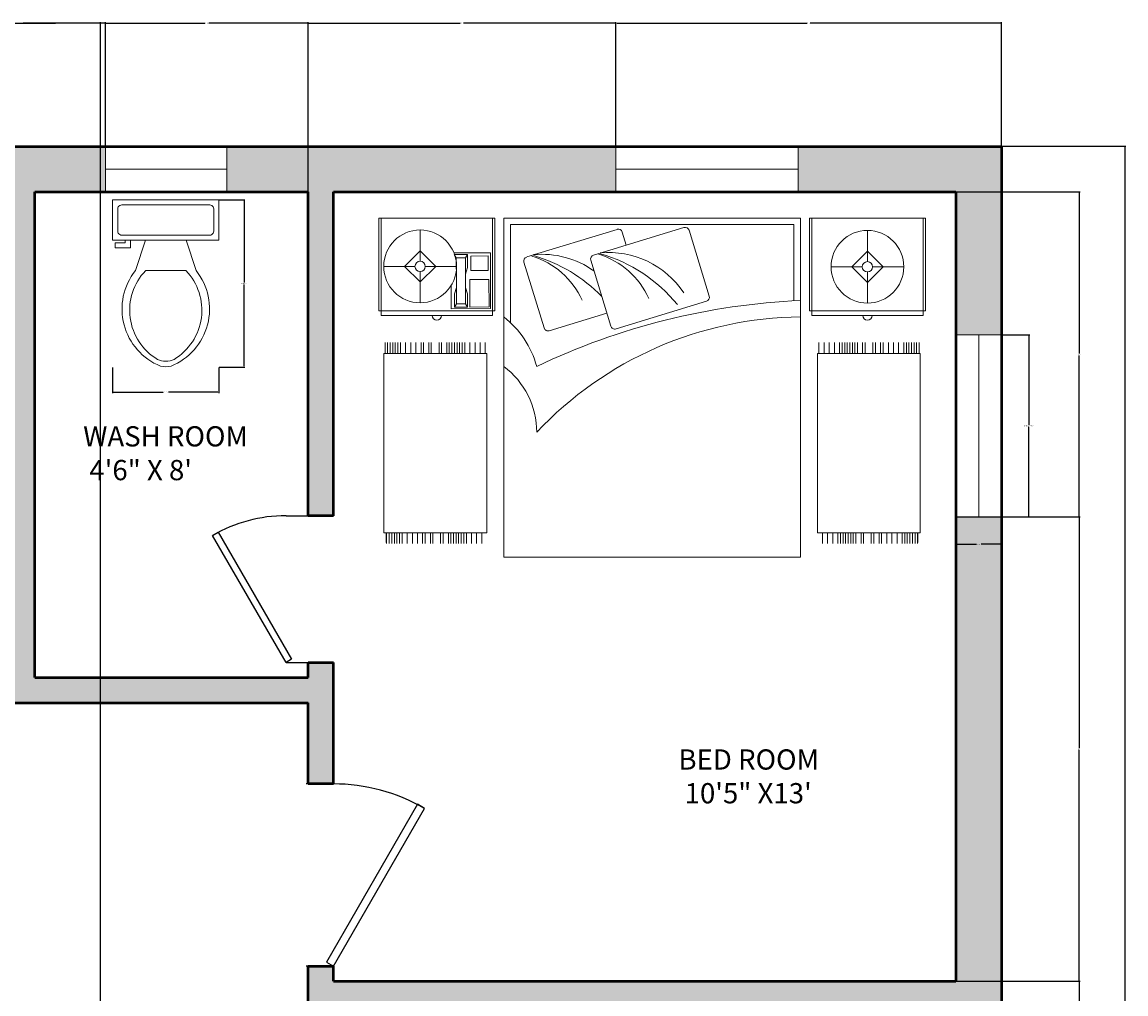
# Model space of a CAD drawing. Units: inches. Extents: x -23 to 411, y -22 to 507.
# Tile 5 of 5: x 193 to 411, y 315 to 507. Entities that reach past the tile are written whole.
import ezdxf

# ---------------------------------------------------------------- set-up
doc = ezdxf.new("R2010")
doc.units = ezdxf.units.IN
doc.header["$MEASUREMENT"] = 0
for name, color, linetype, lineweight in [('A-ANNO-DIMS', 2, 'Continuous', 18), ('A-AREA-IDEN', 7, 'Continuous', 25), ('A-FLOR-FIXT', 90, 'Continuous', 18), ('A-WALL', 7, 'Continuous', 50), ('doors', 40, 'Continuous', 25), ('furniture', 220, 'Continuous', 18), ('window', 30, 'Continuous', 18)]:
    doc.layers.add(name, color=color, linetype=linetype, lineweight=lineweight)
doc.layers.add('A-WALL-PATT', color=179, linetype='Continuous', lineweight=13, true_color=0x161b4b)
doc.styles.get("Standard").update_dxf_attribs({"font": 'arial.ttf'})
doc.dimstyles.get("Standard").update_dxf_attribs({"dimtxt": 0.18, "dimasz": 0.18, "dimexe": 0.18, "dimexo": 0.0625, "dimgap": 0.09, "dimtad": 0, "dimtih": 1, "dimtoh": 1, "dimdec": 4, "dimzin": 0, "dimdsep": 46, "dimtxsty": 'Standard', "dimcen": 0.09, "dimadec": 0, "dimazin": 0, "dimtfac": 1, "dimtdec": 4, "dimtofl": 0, "dimtmove": 0, "dimatfit": 3, "dimfxl": 1, "dimtolj": 1, "dimtzin": 0, "dimarcsym": 0})

# ---------------------------------------------------------------- blocks, each defined once
blk = doc.blocks.new('*U6')
for p, q in [((0, 0), (0, -6)), ((40, 0), (40, -6))]:
    blk.add_line(p, q)
blk.add_lwpolyline([(0, 0), (34.64, 20), (35.52, 18.48), (0.87, -1.52)], close=True)
blk.add_arc((0, 0), 40, 0, 30)
blk = doc.blocks.new('*U7')
for p, q in [((0, 0), (0, 6)), ((40, 0), (40, 6))]:
    blk.add_line(p, q)
blk.add_lwpolyline([(0, 0), (34.64, -20), (35.52, -18.48), (0.87, 1.52)], close=True)
blk.add_arc((0, 0), 40, 330, 0)
blk = doc.blocks.new('3')
for p, q in [((185.8665, 224.6766), (185.8665, 225.2363)), ((185.8665, 225.2363), (186.566, 225.2363)), ((185.8805, 224.6487), (185.8805, 225.2363)), ((186.552, 225.2363), (186.552, 224.6487)), ((186.566, 225.2363), (186.566, 224.6766)), ((186.6199, 225.2363), (186.6199, 224.6399)), ((188.4089, 225.2363), (186.6199, 225.2363)), ((188.4089, 224.7393), (188.4089, 225.2363)), ((188.4627, 225.2363), (188.4627, 224.6766)), ((189.1623, 225.2363), (188.4627, 225.2363)), ((188.4767, 225.2363), (188.4767, 224.6486)), ((189.1483, 224.6486), (189.1483, 225.2363)), ((189.1623, 224.6766), (189.1623, 225.2363)), ((186.1157, 225.1643), (186.1157, 224.9763)), ((187.3034, 225.1683), (186.7581, 225.0015)), ((187.7059, 225.1793), (187.1607, 225.0124)), ((187.3344, 225.1518), (187.3586, 225.073)), ((187.737, 225.1628), (187.8585, 224.7657)), ((188.8125, 225.1618), (188.8125, 224.9738)), ((186.0216, 224.9449), (186.1157, 225.0389)), ((186.1157, 225.0389), (186.2097, 224.9449)), ((186.5397, 225.0274), (186.3193, 225.0266)), ((186.3215, 225.0167), (186.4008, 225.017)), ((186.3334, 224.9969), (186.3215, 225.0167)), ((186.4008, 225.017), (186.389, 224.9971)), ((186.4008, 225.017), (186.4011, 224.9376)), ((186.5409, 224.6901), (186.5397, 225.0274)), ((188.8125, 225.0365), (188.7185, 224.9424)), ((188.9065, 224.9424), (188.8125, 225.0365)), ((186.0843, 224.9449), (185.8963, 224.9449)), ((186.1157, 224.8509), (186.0216, 224.9449)), ((186.2097, 224.9449), (186.1157, 224.8509)), ((186.147, 224.9449), (186.335, 224.9449)), ((186.3334, 224.9969), (186.389, 224.9971)), ((186.334, 224.858), (186.3334, 224.9969)), ((186.3895, 224.8582), (186.389, 224.9971)), ((186.7416, 224.9704), (186.8631, 224.5734)), ((187.1442, 224.9814), (187.2657, 224.5843)), ((186.1157, 224.9136), (186.1157, 224.7256)), ((186.3314, 224.9055), (186.3338, 224.8977)), ((186.4011, 224.9376), (186.3894, 224.8979)), ((188.7812, 224.9424), (188.5931, 224.9424)), ((188.7185, 224.9424), (188.8125, 224.8484)), ((188.8125, 224.8484), (188.9065, 224.9424)), ((188.8125, 224.9111), (188.8125, 224.723)), ((188.8438, 224.9424), (189.0319, 224.9424)), ((186.3023, 224.8297), (186.3029, 224.6892)), ((186.3224, 224.7786), (186.3341, 224.8183)), ((186.334, 224.858), (186.3345, 224.7191)), ((186.3895, 224.8582), (186.39, 224.7193)), ((186.4017, 224.7789), (186.3897, 224.8185)), ((186.3227, 224.6992), (186.3224, 224.7786)), ((186.402, 224.6995), (186.4017, 224.7789)), ((186.3029, 224.6892), (186.5409, 224.6901)), ((186.3345, 224.7191), (186.3227, 224.6992)), ((186.3227, 224.6992), (186.402, 224.6995)), ((186.3345, 224.7191), (186.39, 224.7193)), ((186.402, 224.6995), (186.39, 224.7193)), ((187.842, 224.7347), (187.2967, 224.5678)), ((188.4089, 224.7393), (188.4089, 223.1907)), ((186.566, 224.6766), (185.8665, 224.6766)), ((186.552, 224.6487), (185.8805, 224.6487)), ((186.6199, 224.6399), (186.6199, 223.1907)), ((187.2416, 224.6632), (186.8942, 224.5569)), ((188.4627, 224.6766), (189.1623, 224.6766)), ((188.4767, 224.6486), (189.1483, 224.6486)), ((185.904, 224.4849, -0.9094), (185.904, 224.4204, -0.9094)), ((185.9195, 224.4849, -0.9094), (185.9195, 224.4204, -0.9094)), ((185.9195, 224.4849, -0.9094), (185.9195, 224.4204, -0.9094)), ((185.935, 224.4849, -0.9094), (185.935, 224.4204, -0.9094)), ((185.9505, 224.4849, -0.9094), (185.9505, 224.4204, -0.9094)), ((185.966, 224.4849, -0.9094), (185.966, 224.4204, -0.9094)), ((185.9815, 224.4849, -0.9094), (185.9815, 224.4204, -0.9094)), ((185.997, 224.4849, -0.9094), (185.997, 224.4204, -0.9094)), ((186.028, 224.4849, -0.9094), (186.028, 224.4204, -0.9094)), ((186.059, 224.4849, -0.9094), (186.059, 224.4204, -0.9094)), ((186.09, 224.4849, -0.9094), (186.09, 224.4204, -0.9094)), ((186.09, 224.4849, -0.9094), (186.09, 224.4204, -0.9094)), ((186.121, 224.4849, -0.9094), (186.121, 224.4204, -0.9094)), ((186.1365, 224.4849, -0.9094), (186.1365, 224.4204, -0.9094)), ((186.1675, 224.4849, -0.9094), (186.1675, 224.4204, -0.9094)), ((186.183, 224.4849, -0.9094), (186.183, 224.4204, -0.9094)), ((186.2295, 224.4849, -0.9094), (186.2295, 224.4204, -0.9094)), ((186.245, 224.4849, -0.9094), (186.245, 224.4204, -0.9094)), ((186.276, 224.4849, -0.9094), (186.276, 224.4204, -0.9094)), ((186.2915, 224.4849, -0.9094), (186.2915, 224.4204, -0.9094)), ((186.307, 224.4849, -0.9094), (186.307, 224.4204, -0.9094)), ((186.3225, 224.4849, -0.9094), (186.3225, 224.4204, -0.9094)), ((186.338, 224.4849, -0.9094), (186.338, 224.4204, -0.9094)), ((186.3535, 224.4849, -0.9094), (186.3535, 224.4204, -0.9094)), ((186.369, 224.4849, -0.9094), (186.369, 224.4204, -0.9094)), ((186.3845, 224.4849, -0.9094), (186.3845, 224.4204, -0.9094)), ((186.4155, 224.4849, -0.9094), (186.4155, 224.4204, -0.9094)), ((186.4465, 224.4849, -0.9094), (186.4465, 224.4204, -0.9094)), ((186.4775, 224.4849, -0.9094), (186.4775, 224.4204, -0.9094)), ((186.5085, 224.4849, -0.9094), (186.5085, 224.4204, -0.9094)), ((188.5202, 224.4849, -0.9094), (188.5202, 224.4204, -0.9094)), ((188.5512, 224.4849, -0.9094), (188.5512, 224.4204, -0.9094)), ((188.5822, 224.4849, -0.9094), (188.5822, 224.4204, -0.9094)), ((188.6132, 224.4849, -0.9094), (188.6132, 224.4204, -0.9094)), ((188.6442, 224.4849, -0.9094), (188.6442, 224.4204, -0.9094)), ((188.6597, 224.4849, -0.9094), (188.6597, 224.4204, -0.9094)), ((188.6752, 224.4849, -0.9094), (188.6752, 224.4204, -0.9094)), ((188.6907, 224.4849, -0.9094), (188.6907, 224.4204, -0.9094)), ((188.7062, 224.4849, -0.9094), (188.7062, 224.4204, -0.9094)), ((188.7217, 224.4849, -0.9094), (188.7217, 224.4204, -0.9094)), ((188.7372, 224.4849, -0.9094), (188.7372, 224.4204, -0.9094)), ((188.7527, 224.4849, -0.9094), (188.7527, 224.4204, -0.9094)), ((188.7837, 224.4849, -0.9094), (188.7837, 224.4204, -0.9094)), ((188.7992, 224.4849, -0.9094), (188.7992, 224.4204, -0.9094)), ((188.8457, 224.4849, -0.9094), (188.8457, 224.4204, -0.9094)), ((188.8612, 224.4849, -0.9094), (188.8612, 224.4204, -0.9094)), ((188.8922, 224.4849, -0.9094), (188.8922, 224.4204, -0.9094)), ((188.9077, 224.4849, -0.9094), (188.9077, 224.4204, -0.9094)), ((188.9387, 224.4849, -0.9094), (188.9387, 224.4204, -0.9094)), ((188.9387, 224.4849, -0.9094), (188.9387, 224.4204, -0.9094)), ((188.9697, 224.4849, -0.9094), (188.9697, 224.4204, -0.9094)), ((189.0007, 224.4849, -0.9094), (189.0007, 224.4204, -0.9094)), ((189.0317, 224.4849, -0.9094), (189.0317, 224.4204, -0.9094)), ((189.0472, 224.4849, -0.9094), (189.0472, 224.4204, -0.9094)), ((189.0627, 224.4849, -0.9094), (189.0627, 224.4204, -0.9094)), ((189.0782, 224.4849, -0.9094), (189.0782, 224.4204, -0.9094)), ((189.0937, 224.4849, -0.9094), (189.0937, 224.4204, -0.9094)), ((189.1092, 224.4849, -0.9094), (189.1092, 224.4204, -0.9094)), ((189.1092, 224.4849, -0.9094), (189.1092, 224.4204, -0.9094)), ((189.1247, 224.4849, -0.9094), (189.1247, 224.4204, -0.9094)), ((185.8974, 224.4204, -0.9094), (185.8974, 223.3378, -0.9094)), ((185.8974, 224.4204, -0.9094), (186.5174, 224.4204, -0.9094)), ((186.5174, 224.4204, -0.9094), (186.5174, 223.3378, -0.9094)), ((189.1313, 224.4204, -0.9094), (188.5113, 224.4204, -0.9094)), ((188.5113, 224.4204, -0.9094), (188.5113, 223.3378, -0.9094)), ((189.1313, 224.4204, -0.9094), (189.1313, 223.3378, -0.9094)), ((185.8974, 223.3378, -0.9094), (186.5174, 223.3378, -0.9094)), ((185.9114, 223.3378, -0.9094), (185.9114, 223.2789, -0.9094)), ((185.9114, 223.3378, -0.9094), (185.9114, 223.2789, -0.9094)), ((185.9114, 223.3378, -0.9094), (185.9114, 223.2789, -0.9094)), ((185.9138, 223.3378, -0.9094), (185.9138, 223.2732, -0.9094)), ((185.9293, 223.3378, -0.9094), (185.9293, 223.2732, -0.9094)), ((185.9293, 223.3378, -0.9094), (185.9293, 223.2732, -0.9094)), ((185.9448, 223.3378, -0.9094), (185.9448, 223.2732, -0.9094)), ((185.9603, 223.3378, -0.9094), (185.9603, 223.2732, -0.9094)), ((185.9758, 223.3378, -0.9094), (185.9758, 223.2732, -0.9094)), ((185.9913, 223.3378, -0.9094), (185.9913, 223.2732, -0.9094)), ((186.0068, 223.3378, -0.9094), (186.0068, 223.2732, -0.9094)), ((186.0378, 223.3378, -0.9094), (186.0378, 223.2732, -0.9094)), ((186.0688, 223.3378, -0.9094), (186.0688, 223.2732, -0.9094)), ((186.0998, 223.3378, -0.9094), (186.0998, 223.2732, -0.9094)), ((186.0998, 223.3378, -0.9094), (186.0998, 223.2732, -0.9094)), ((186.1308, 223.3378, -0.9094), (186.1308, 223.2732, -0.9094)), ((186.1463, 223.3378, -0.9094), (186.1463, 223.2732, -0.9094)), ((186.1773, 223.3378, -0.9094), (186.1773, 223.2732, -0.9094)), ((186.1928, 223.3378, -0.9094), (186.1928, 223.2732, -0.9094)), ((186.2393, 223.3378, -0.9094), (186.2393, 223.2732, -0.9094)), ((186.2548, 223.3378, -0.9094), (186.2548, 223.2732, -0.9094)), ((186.2858, 223.3378, -0.9094), (186.2858, 223.2732, -0.9094)), ((186.3013, 223.3378, -0.9094), (186.3013, 223.2732, -0.9094)), ((186.3168, 223.3378, -0.9094), (186.3168, 223.2732, -0.9094)), ((186.3323, 223.3378, -0.9094), (186.3323, 223.2732, -0.9094)), ((186.3478, 223.3378, -0.9094), (186.3478, 223.2732, -0.9094)), ((186.3633, 223.3378, -0.9094), (186.3633, 223.2732, -0.9094)), ((186.3788, 223.3378, -0.9094), (186.3788, 223.2732, -0.9094)), ((186.3943, 223.3378, -0.9094), (186.3943, 223.2732, -0.9094)), ((186.4253, 223.3378, -0.9094), (186.4253, 223.2732, -0.9094)), ((186.4563, 223.3378, -0.9094), (186.4563, 223.2732, -0.9094)), ((186.4873, 223.3378, -0.9094), (186.4873, 223.2732, -0.9094)), ((189.1313, 223.3378, -0.9094), (188.5113, 223.3378, -0.9094)), ((188.5414, 223.3378, -0.9094), (188.5414, 223.2732, -0.9094)), ((188.5724, 223.3378, -0.9094), (188.5724, 223.2732, -0.9094)), ((188.6034, 223.3378, -0.9094), (188.6034, 223.2732, -0.9094)), ((188.6344, 223.3378, -0.9094), (188.6344, 223.2732, -0.9094)), ((188.6499, 223.3378, -0.9094), (188.6499, 223.2732, -0.9094)), ((188.6654, 223.3378, -0.9094), (188.6654, 223.2732, -0.9094)), ((188.6809, 223.3378, -0.9094), (188.6809, 223.2732, -0.9094)), ((188.6964, 223.3378, -0.9094), (188.6964, 223.2732, -0.9094)), ((188.7119, 223.3378, -0.9094), (188.7119, 223.2732, -0.9094)), ((188.7274, 223.3378, -0.9094), (188.7274, 223.2732, -0.9094)), ((188.7429, 223.3378, -0.9094), (188.7429, 223.2732, -0.9094)), ((188.7739, 223.3378, -0.9094), (188.7739, 223.2732, -0.9094)), ((188.7894, 223.3378, -0.9094), (188.7894, 223.2732, -0.9094)), ((188.8359, 223.3378, -0.9094), (188.8359, 223.2732, -0.9094)), ((188.8514, 223.3378, -0.9094), (188.8514, 223.2732, -0.9094)), ((188.8824, 223.3378, -0.9094), (188.8824, 223.2732, -0.9094)), ((188.8979, 223.3378, -0.9094), (188.8979, 223.2732, -0.9094)), ((188.9289, 223.3378, -0.9094), (188.9289, 223.2732, -0.9094)), ((188.9289, 223.3378, -0.9094), (188.9289, 223.2732, -0.9094)), ((188.9599, 223.3378, -0.9094), (188.9599, 223.2732, -0.9094)), ((188.9909, 223.3378, -0.9094), (188.9909, 223.2732, -0.9094)), ((189.022, 223.3378, -0.9094), (189.022, 223.2732, -0.9094)), ((189.0375, 223.3378, -0.9094), (189.0375, 223.2732, -0.9094)), ((189.053, 223.3378, -0.9094), (189.053, 223.2732, -0.9094)), ((189.0685, 223.3378, -0.9094), (189.0685, 223.2732, -0.9094)), ((189.084, 223.3378, -0.9094), (189.084, 223.2732, -0.9094)), ((189.0995, 223.3378, -0.9094), (189.0995, 223.2732, -0.9094)), ((189.0995, 223.3378, -0.9094), (189.0995, 223.2732, -0.9094)), ((189.115, 223.3378, -0.9094), (189.115, 223.2732, -0.9094)), ((189.1173, 223.3378, -0.9094), (189.1173, 223.2789, -0.9094)), ((189.1173, 223.3378, -0.9094), (189.1173, 223.2789, -0.9094)), ((189.1173, 223.3378, -0.9094), (189.1173, 223.2789, -0.9094)), ((186.6199, 223.1907), (188.4089, 223.1907))]:
    blk.add_line(p, q)
blk.add_lwpolyline([(188.3691, 224.7374), (188.3691, 225.1965), (186.6596, 225.1965), (186.6596, 224.606)])
for points in [[(186.4217, 225.0072), (186.422, 224.9199), (186.5252, 224.9202), (186.5249, 225.0075)], [(186.4153, 224.8663), (186.4159, 224.6996), (186.531, 224.7), (186.5304, 224.8667)]]:
    blk.add_lwpolyline(points, close=True)
for points in [[(186.6199, 224.6399, -0.162278), (186.8186, 224.3418, -0.100664), (188.4089, 224.7393, -0.100664)], [(186.6199, 224.3418, -0.236068), (186.8186, 223.9442, -0.205258), (188.4089, 224.6399, -0.205258)]]:
    blk.add_lwpolyline(points, format="xyb")
for centre, radius in [((186.1157, 224.9449), 0.2194), ((188.8125, 224.9424), 0.2194), ((186.1157, 224.9449), 0.0313), ((188.8125, 224.9424), 0.0313)]:
    blk.add_circle(centre, radius)
for centre, radius, start, end in [((187.3107, 225.1446), 0.0248, 17.0142, 107.0142), ((187.7132, 225.1555), 0.0248, 17.0142, 107.0142), ((186.8477, 224.4712), 0.5468, 54.68511, 95.16051), ((187.1679, 224.9887), 0.0248, 107.0142, 197.0142), ((187.0499, 224.5517), 0.4873, 24.22087, 73.06906), ((187.2502, 224.4821), 0.5468, 33.78007, 95.16051), ((186.9385, 224.1164), 0.9426, 39.40233, 73.71889), ((186.7654, 224.9777), 0.0248, 107.0142, 197.0142), ((186.6474, 224.5408), 0.4873, 24.22087, 73.06906), ((186.5359, 224.1054), 0.9426, 44.27274, 73.71889), ((187.8347, 224.7585), 0.0248, 287.0142, 17.0142), ((186.2163, 224.6487), 0.028, 180, 0), ((188.8125, 224.6486), 0.028, 180, 0), ((186.8869, 224.5806), 0.0248, 197.0142, 287.0142), ((187.2894, 224.5916), 0.0248, 197.0142, 287.0142)]:
    blk.add_arc(centre, radius, start, end)
blk = doc.blocks.new('Toilet - top')
for p, q in [((9.5, -6), (9.5, -2)), ((-10, -8.5), (-8, -8.5)), ((-10, -9.5), (-10, -8.5)), ((-8, -8.5), (-8, -8)), ((-7, -8), (-7, -9.5)), ((-4, -8), (-6, -14)), ((4, -8), (6, -14)), ((-7, -9.5), (-10, -9.5)), ((4, -14), (-4, -14))]:
    blk.add_line(p, q)
blk.add_lwpolyline([(10.5, -8), (10.5, 0), (-10.5, 0), (-10.5, -8)], close=True)
for points in [[(-9.5, -2), (-9.5, -6)], [(8.5, -1), (-8.5, -1)], [(-8.5, -7), (8.5, -7)]]:
    blk.add_lwpolyline(points)
for centre, radius, start, end in [((-8.62, -1.88), 0.884, 81.8699, 188.1301), ((8.62, -1.88), 0.884, 351.8699, 98.1301), ((-8.62, -6.12), 0.884, 171.8699, 278.1301), ((8.62, -6.12), 0.884, 261.8699, 8.1301), ((3.52, -21.58), 12.17, 141.4691, 247.9714), ((4.2, -21.82), 11.33, 136.3677, 238.9468), ((-3.52, -21.58), 12.17, 292.0284, 38.5307), ((-4.2, -21.82), 11.33, 301.053, 43.6321), ((0, -27.88), 4, 245.7318, 294.2682), ((0, -29), 4, 254.8605, 285.1395)]:
    blk.add_arc(centre, radius, start, end)
blk = doc.blocks.new('WIN-36IN')
for p, q in [((9, 36), (0, 36)), ((0, 36), (0, 0)), ((4.5, 0), (4.5, 36)), ((9, 0), (9, 36)), ((0, 0), (9, 0)), ((0, 0), (4.5, 0))]:
    blk.add_line(p, q)
blk = doc.blocks.new('WIN-24IN')
for p, q in [((0, 9), (0, 0)), ((24, 9), (0, 9)), ((0, 9), (0, 4.5)), ((24, 0), (24, 9)), ((0, 4.5), (24, 4.5)), ((0, 0), (24, 0))]:
    blk.add_line(p, q)
blk = doc.blocks.new('*D12')
at = {"layer": 'A-ANNO-DIMS', "color": 0, "lineweight": -2, "transparency": 16777216}
for p, q in [((386.24, 445.65), (391.75, 445.65)), ((391.57, 445.47), (391.57, 427.83)), ((391.57, 409.83), (391.57, 427.46)), ((386.24, 409.65), (391.75, 409.65))]:
    blk.add_line(p, q, dxfattribs=at)
at = {"layer": 'A-ANNO-DIMS', "color": 0, "transparency": 16777216}
for points in [[(391.54, 445.47), (391.6, 445.47), (391.57, 445.65)], [(391.54, 409.83), (391.6, 409.83), (391.57, 409.65)]]:
    blk.add_solid(points, dxfattribs=at)
at = {"layer": 'Defpoints', "color": 0, "transparency": 16777216}
for p in [(386.17, 445.65), (391.57, 445.65), (386.17, 409.65)]:
    blk.add_point(p, dxfattribs=at)
at = {"layer": 'A-ANNO-DIMS', "color": 0, "transparency": 16777216, "insert": (391.57, 427.65), "char_height": 0.18, "attachment_point": 5}
blk.add_mtext('\\A1;WINDOW 36 TYP.', dxfattribs=at)
blk = doc.blocks.new('*D13')
at = {"layer": 'A-ANNO-DIMS', "color": 0, "lineweight": -2, "transparency": 16777216}
for p, q in [((377.17, 409.58), (377.17, 404.07)), ((386.17, 409.58), (386.17, 404.07)), ((377.35, 404.25), (381.22, 404.25)), ((385.99, 404.25), (382.13, 404.25))]:
    blk.add_line(p, q, dxfattribs=at)
at = {"layer": 'A-ANNO-DIMS', "color": 0, "transparency": 16777216}
for points in [[(377.35, 404.28), (377.35, 404.22), (377.17, 404.25)], [(385.99, 404.28), (385.99, 404.22), (386.17, 404.25)]]:
    blk.add_solid(points, dxfattribs=at)
at = {"layer": 'Defpoints', "color": 0, "transparency": 16777216}
for p in [(377.17, 409.65), (386.17, 409.65), (386.17, 404.25)]:
    blk.add_point(p, dxfattribs=at)
at = {"layer": 'A-ANNO-DIMS', "color": 0, "transparency": 16777216, "insert": (381.67, 404.25), "char_height": 0.18, "attachment_point": 5}
blk.add_mtext('\\A1;9 TYP.', dxfattribs=at)
blk = doc.blocks.new('*D18')
at = {"layer": 'A-ANNO-DIMS', "color": 0, "lineweight": -2, "transparency": 16777216}
for p, q in [((231.63, 472.33), (236.7, 472.33)), ((236.52, 472.15), (236.52, 455.99)), ((236.52, 439.46), (236.52, 455.62)), ((231.63, 439.28), (236.7, 439.28))]:
    blk.add_line(p, q, dxfattribs=at)
at = {"layer": 'A-ANNO-DIMS', "color": 0, "transparency": 16777216}
for points in [[(236.49, 472.15), (236.55, 472.15), (236.52, 472.33)], [(236.49, 439.46), (236.55, 439.46), (236.52, 439.28)]]:
    blk.add_solid(points, dxfattribs=at)
at = {"layer": 'Defpoints', "color": 0, "transparency": 16777216}
for p in [(231.56, 472.33), (236.52, 472.33), (231.56, 439.28)]:
    blk.add_point(p, dxfattribs=at)
at = {"layer": 'A-ANNO-DIMS', "color": 0, "transparency": 16777216, "insert": (236.52, 455.8), "char_height": 0.18, "attachment_point": 5}
blk.add_mtext('\\A1;WC 33 TYP.', dxfattribs=at)
blk = doc.blocks.new('*D19')
at = {"layer": 'A-ANNO-DIMS', "color": 0, "lineweight": -2, "transparency": 16777216}
for p, q in [((210.56, 439.22), (210.56, 434.14)), ((231.56, 439.22), (231.56, 434.14)), ((210.74, 434.32), (220.53, 434.32)), ((231.38, 434.32), (221.59, 434.32))]:
    blk.add_line(p, q, dxfattribs=at)
at = {"layer": 'A-ANNO-DIMS', "color": 0, "transparency": 16777216}
for points in [[(210.74, 434.35), (210.74, 434.29), (210.56, 434.32)], [(231.38, 434.35), (231.38, 434.29), (231.56, 434.32)]]:
    blk.add_solid(points, dxfattribs=at)
at = {"layer": 'Defpoints', "color": 0, "transparency": 16777216}
for p in [(210.56, 439.28), (231.56, 439.28), (231.56, 434.32)]:
    blk.add_point(p, dxfattribs=at)
at = {"layer": 'A-ANNO-DIMS', "color": 0, "transparency": 16777216, "insert": (221.06, 434.32), "char_height": 0.18, "attachment_point": 5}
blk.add_mtext('\\A1;21 TYP.', dxfattribs=at)
blk = doc.blocks.new('*D29')
at = {"layer": 'A-ANNO-DIMS', "color": 0, "lineweight": -2, "transparency": 16777216}
for p, q in [((386.24, 482.9), (410.73, 482.9)), ((410.55, 482.72), (410.55, 243.08)), ((410.55, 3.08), (410.55, 242.72)), ((386.24, 2.9), (410.73, 2.9))]:
    blk.add_line(p, q, dxfattribs=at)
at = {"layer": 'A-ANNO-DIMS', "color": 0, "transparency": 16777216}
for points in [[(410.52, 482.72), (410.58, 482.72), (410.55, 482.9)], [(410.52, 3.08), (410.58, 3.08), (410.55, 2.9)]]:
    blk.add_solid(points, dxfattribs=at)
at = {"layer": 'Defpoints', "color": 0, "transparency": 16777216}
for p in [(386.17, 482.9), (386.17, 2.9), (410.55, 2.9)]:
    blk.add_point(p, dxfattribs=at)
at = {"layer": 'A-ANNO-DIMS', "color": 0, "transparency": 16777216, "insert": (410.55, 242.9), "char_height": 0.18, "attachment_point": 5}
blk.add_mtext('\\A1;480', dxfattribs=at)
blk = doc.blocks.new('*D34')
at = {"layer": 'A-ANNO-DIMS', "color": 0, "lineweight": -2, "transparency": 16777216}
for p, q in [((190.17, 473.96), (190.17, 507.45)), ((190.35, 507.27), (199.27, 507.27)), ((208.96, 507.27), (200.04, 507.27)), ((209.14, 482.96), (209.14, 507.45))]:
    blk.add_line(p, q, dxfattribs=at)
at = {"layer": 'A-ANNO-DIMS', "color": 0, "transparency": 16777216}
for points in [[(190.35, 507.3), (190.35, 507.24), (190.17, 507.27)], [(208.96, 507.3), (208.96, 507.24), (209.14, 507.27)]]:
    blk.add_solid(points, dxfattribs=at)
at = {"layer": 'Defpoints', "color": 0, "transparency": 16777216}
for p in [(209.14, 507.27), (209.14, 482.9), (190.17, 473.9)]:
    blk.add_point(p, dxfattribs=at)
at = {"layer": 'A-ANNO-DIMS', "color": 0, "transparency": 16777216, "insert": (199.66, 507.27), "char_height": 0.18, "attachment_point": 5}
blk.add_mtext('\\A1;18.96', dxfattribs=at)
blk = doc.blocks.new('*D35')
at = {"layer": 'A-ANNO-DIMS', "color": 0, "lineweight": -2, "transparency": 16777216}
for p, q in [((209.14, 482.96), (209.14, 507.45)), ((209.32, 507.27), (228.76, 507.27)), ((248.99, 507.27), (229.55, 507.27)), ((249.17, 473.96), (249.17, 507.45))]:
    blk.add_line(p, q, dxfattribs=at)
at = {"layer": 'A-ANNO-DIMS', "color": 0, "transparency": 16777216}
for points in [[(209.32, 507.3), (209.32, 507.24), (209.14, 507.27)], [(248.99, 507.3), (248.99, 507.24), (249.17, 507.27)]]:
    blk.add_solid(points, dxfattribs=at)
at = {"layer": 'Defpoints', "color": 0, "transparency": 16777216}
for p in [(249.17, 507.27), (209.14, 482.9), (249.17, 473.9)]:
    blk.add_point(p, dxfattribs=at)
at = {"layer": 'A-ANNO-DIMS', "color": 0, "transparency": 16777216, "insert": (229.16, 507.27), "char_height": 0.18, "attachment_point": 5}
blk.add_mtext('\\A1;40.04', dxfattribs=at)
blk = doc.blocks.new('*D36')
at = {"layer": 'A-ANNO-DIMS', "color": 0, "lineweight": -2, "transparency": 16777216}
for p, q in [((249.17, 473.96), (249.17, 507.45)), ((249.35, 507.27), (279.25, 507.27)), ((309.79, 507.27), (279.9, 507.27)), ((309.97, 482.96), (309.97, 507.45))]:
    blk.add_line(p, q, dxfattribs=at)
at = {"layer": 'A-ANNO-DIMS', "color": 0, "transparency": 16777216}
for points in [[(249.35, 507.3), (249.35, 507.24), (249.17, 507.27)], [(309.79, 507.3), (309.79, 507.24), (309.97, 507.27)]]:
    blk.add_solid(points, dxfattribs=at)
at = {"layer": 'Defpoints', "color": 0, "transparency": 16777216}
for p in [(309.97, 507.27), (309.97, 482.9), (249.17, 473.9)]:
    blk.add_point(p, dxfattribs=at)
at = {"layer": 'A-ANNO-DIMS', "color": 0, "transparency": 16777216, "insert": (279.57, 507.27), "char_height": 0.18, "attachment_point": 5}
blk.add_mtext('\\A1;60.8', dxfattribs=at)
blk = doc.blocks.new('*D37')
at = {"layer": 'A-ANNO-DIMS', "color": 0, "lineweight": -2, "transparency": 16777216}
for p, q in [((309.97, 482.96), (309.97, 507.45)), ((310.15, 507.27), (347.75, 507.27)), ((385.99, 507.27), (348.4, 507.27)), ((386.17, 482.96), (386.17, 507.45))]:
    blk.add_line(p, q, dxfattribs=at)
at = {"layer": 'A-ANNO-DIMS', "color": 0, "transparency": 16777216}
for points in [[(310.15, 507.3), (310.15, 507.24), (309.97, 507.27)], [(385.99, 507.3), (385.99, 507.24), (386.17, 507.27)]]:
    blk.add_solid(points, dxfattribs=at)
at = {"layer": 'Defpoints', "color": 0, "transparency": 16777216}
for p in [(386.17, 507.27), (309.97, 482.9), (386.17, 482.9)]:
    blk.add_point(p, dxfattribs=at)
at = {"layer": 'A-ANNO-DIMS', "color": 0, "transparency": 16777216, "insert": (348.07, 507.27), "char_height": 0.18, "attachment_point": 5}
blk.add_mtext('\\A1;76.2', dxfattribs=at)
blk = doc.blocks.new('*D46')
at = {"layer": 'A-ANNO-DIMS', "color": 0, "lineweight": -2, "transparency": 16777216}
for p, q in [((177.17, 107.96), (177.17, 507.45)), ((177.35, 507.27), (192.47, 507.27)), ((207.99, 507.27), (192.88, 507.27)), ((208.17, 107.96), (208.17, 507.45))]:
    blk.add_line(p, q, dxfattribs=at)
at = {"layer": 'A-ANNO-DIMS', "color": 0, "transparency": 16777216}
for points in [[(177.35, 507.3), (177.35, 507.24), (177.17, 507.27)], [(207.99, 507.3), (207.99, 507.24), (208.17, 507.27)]]:
    blk.add_solid(points, dxfattribs=at)
at = {"layer": 'Defpoints', "color": 0, "transparency": 16777216}
for p in [(208.17, 507.27), (177.17, 107.9), (208.17, 107.9)]:
    blk.add_point(p, dxfattribs=at)
at = {"layer": 'A-ANNO-DIMS', "color": 0, "transparency": 16777216, "insert": (192.67, 507.27), "char_height": 0.18, "attachment_point": 5}
blk.add_mtext('\\A1;31', dxfattribs=at)
blk = doc.blocks.new('*D55')
at = {"layer": 'A-ANNO-DIMS', "color": 0, "lineweight": -2, "transparency": 16777216}
for p, q in [((377.24, 317.9), (401.73, 317.9)), ((401.55, 317.72), (401.55, 281.82)), ((401.55, 245.55), (401.55, 281.45)), ((377.24, 245.37), (401.73, 245.37))]:
    blk.add_line(p, q, dxfattribs=at)
at = {"layer": 'A-ANNO-DIMS', "color": 0, "transparency": 16777216}
for points in [[(401.52, 317.72), (401.58, 317.72), (401.55, 317.9)], [(401.52, 245.55), (401.58, 245.55), (401.55, 245.37)]]:
    blk.add_solid(points, dxfattribs=at)
at = {"layer": 'Defpoints', "color": 0, "transparency": 16777216}
for p in [(377.17, 317.9), (377.17, 245.37), (401.55, 245.37)]:
    blk.add_point(p, dxfattribs=at)
at = {"layer": 'A-ANNO-DIMS', "color": 0, "transparency": 16777216, "insert": (401.55, 281.64), "char_height": 0.18, "attachment_point": 5}
blk.add_mtext('\\A1;72.52', dxfattribs=at)
blk = doc.blocks.new('*D56')
at = {"layer": 'A-ANNO-DIMS', "color": 0, "lineweight": -2, "transparency": 16777216}
for p, q in [((377.24, 409.65), (401.73, 409.65)), ((401.55, 409.47), (401.55, 363.95)), ((401.55, 318.08), (401.55, 363.59)), ((377.24, 317.9), (401.73, 317.9))]:
    blk.add_line(p, q, dxfattribs=at)
at = {"layer": 'A-ANNO-DIMS', "color": 0, "transparency": 16777216}
for points in [[(401.52, 409.47), (401.58, 409.47), (401.55, 409.65)], [(401.52, 318.08), (401.58, 318.08), (401.55, 317.9)]]:
    blk.add_solid(points, dxfattribs=at)
at = {"layer": 'Defpoints', "color": 0, "transparency": 16777216}
for p in [(377.17, 409.65), (377.17, 317.9), (401.55, 317.9)]:
    blk.add_point(p, dxfattribs=at)
at = {"layer": 'A-ANNO-DIMS', "color": 0, "transparency": 16777216, "insert": (401.55, 363.77), "char_height": 0.18, "attachment_point": 5}
blk.add_mtext('\\A1;91.75', dxfattribs=at)
blk = doc.blocks.new('*D57')
at = {"layer": 'A-ANNO-DIMS', "color": 0, "lineweight": -2, "transparency": 16777216}
for p, q in [((377.24, 473.9), (401.73, 473.9)), ((401.55, 473.72), (401.55, 441.95)), ((401.55, 409.83), (401.55, 441.59)), ((377.24, 409.65), (401.73, 409.65))]:
    blk.add_line(p, q, dxfattribs=at)
at = {"layer": 'A-ANNO-DIMS', "color": 0, "transparency": 16777216}
for points in [[(401.52, 473.72), (401.58, 473.72), (401.55, 473.9)], [(401.52, 409.83), (401.58, 409.83), (401.55, 409.65)]]:
    blk.add_solid(points, dxfattribs=at)
at = {"layer": 'Defpoints', "color": 0, "transparency": 16777216}
for p in [(377.17, 473.9), (377.17, 409.65), (401.55, 409.65)]:
    blk.add_point(p, dxfattribs=at)
at = {"layer": 'A-ANNO-DIMS', "color": 0, "transparency": 16777216, "insert": (401.55, 441.77), "char_height": 0.18, "attachment_point": 5}
blk.add_mtext('\\A1;64.25', dxfattribs=at)

msp = doc.modelspace()

# ---------------------------------------------------------------- hatches: boundary and pattern name
at = {"layer": 'A-WALL-PATT'}
h = msp.add_hatch(color=256, dxfattribs=at)
h.dxf.hatch_style = 1
h.paths.add_polyline_path([(37.3453, 482.8972), (2.1746, 482.8972), (2.1746, 414.9823), (11.1746, 414.9823), (11.1746, 473.8972), (37.3453, 473.8972)])
h.paths.add_polyline_path([(149.2817, 482.8972), (73.3453, 482.8972), (73.3453, 473.8972), (131.1746, 473.8972), (131.1746, 356.8972), (136.1746, 356.8972), (136.1746, 372.8972), (139.1746, 372.8972), (139.1746, 377.8972), (136.1746, 377.8972), (136.1746, 473.8972), (149.2817, 473.8972)])
h.paths.add_polyline_path([(209.1361, 482.8972), (173.2817, 482.8972), (173.2817, 473.8972), (190.1746, 473.8972), (190.1746, 377.8972), (168.1746, 377.8972), (168.1746, 372.8972), (249.1746, 372.8972), (249.1746, 356.8972), (254.1746, 356.8972), (254.1746, 380.8972), (249.1746, 380.8972), (249.1746, 377.8972), (195.1746, 377.8972), (195.1746, 473.8972), (209.1361, 473.8972)])
h.paths.add_polyline_path([(309.9724, 482.8972), (233.1361, 482.8972), (233.1361, 473.8972), (249.1746, 473.8972), (249.1746, 409.8972), (254.1746, 409.8972), (254.1746, 473.8972), (309.9724, 473.8972)])
h.paths.add_polyline_path([(386.1746, 482.8972), (345.9724, 482.8972), (345.9724, 473.8972), (377.1746, 473.8972), (377.1746, 445.6454), (386.1746, 445.6454)])
h.paths.add_polyline_path([(386.1746, 409.6454), (377.1746, 409.6454), (377.1746, 317.8972), (254.1746, 317.8972), (254.1746, 320.8972), (249.1746, 320.8972), (249.1746, 317.8972), (249.1746, 235.8972), (254.1746, 235.8972), (254.1746, 312.8972), (377.1746, 312.8972), (377.1746, 281.3732), (386.1746, 281.3732)])
h.paths.add_polyline_path([(386.1746, 245.3732), (377.1746, 245.3732), (377.1746, 196.8972), (254.1746, 196.8972), (254.1746, 199.8972), (249.1746, 199.8972), (249.1746, 196.8972), (249.1746, 188.8972), (254.1746, 188.8972), (254.1746, 191.8972), (264.1746, 191.8972), (377.1746, 191.8972), (377.1746, 11.8972), (377.1746, 2.8972), (386.1746, 2.8972)])
h.paths.add_polyline_path([(254.1746, 128.8972), (249.1746, 128.8972), (249.1746, 11.8972), (206.9157, 11.8972), (206.9157, 2.8972), (254.1746, 2.8972)])
h.paths.add_polyline_path([(170.9157, 11.8972), (86.2116, 11.8972), (86.2116, 2.8972), (170.9157, 2.8972)])
h.paths.add_polyline_path([(136.1746, 114.8972), (131.1746, 114.8972), (131.1746, 11.8972), (136.1746, 11.8972)])
h.paths.add_polyline_path([(50.2116, 11.8972), (11.1746, 11.8972), (11.1746, 90.1201), (2.1746, 90.1201), (2.1746, 2.8972), (50.2116, 2.8972)])
h.paths.add_polyline_path([(11.1746, 176.2548), (2.1746, 176.2548), (2.1746, 126.1201), (11.1746, 126.1201)])
h.paths.add_polyline_path([(136.1746, 158.8972), (11.1746, 158.8972), (11.1746, 153.8972), (131.1746, 153.8972), (131.1746, 150.8972), (136.1746, 150.8972)])
h.paths.add_polyline_path([(11.1746, 269.5052), (2.1746, 269.5052), (2.1746, 212.2548), (11.1746, 212.2548)])
h.paths.add_polyline_path([(11.1746, 378.9823), (2.1746, 378.9823), (2.1746, 305.5052), (11.1746, 305.5052), (11.1746, 312.8972), (136.1746, 312.8972), (136.1746, 320.8972), (131.1746, 320.8972), (131.1746, 317.8972), (11.1746, 317.8972)])

# ---------------------------------------------------------------- linework, layer by layer
at = {"layer": 'A-WALL'}
for p, q in [((195.1746, 473.8972), (249.1746, 473.8972)), ((195.1746, 377.8972), (195.1746, 473.8972)), ((249.1746, 409.8972), (249.1746, 473.8972)), ((254.1746, 473.8972), (377.1746, 473.8972)), ((254.1746, 409.8972), (254.1746, 473.8972)), ((377.1746, 473.8972), (377.1746, 317.8972)), ((254.1746, 409.8972), (249.1746, 409.8972)), ((249.1746, 377.8972), (249.1746, 380.8972)), ((249.1746, 377.8972), (249.1746, 380.8972)), ((249.1746, 380.8972), (254.1746, 380.8972)), ((254.1746, 356.8972), (254.1746, 380.8972)), ((195.1746, 377.8972), (249.1746, 377.8972)), ((168.1746, 372.8972), (249.1746, 372.8972)), ((249.1746, 356.8972), (249.1746, 372.8972)), ((254.1746, 356.8972), (249.1746, 356.8972)), ((249.1746, 235.8972), (249.1746, 320.8972)), ((249.1746, 317.8972), (249.1746, 320.8972)), ((249.1746, 320.8972), (254.1746, 320.8972)), ((254.1746, 317.8972), (254.1746, 320.8972)), ((254.1746, 317.8972), (377.1746, 317.8972))]:
    msp.add_line(p, q, dxfattribs=at)
msp.add_lwpolyline([(254.1746, 2.8972), (2.1746, 2.8972), (2.1746, 482.8972), (386.1746, 482.8972), (386.1746, 2.8972), (377.1746, 2.8972)], dxfattribs=at)

# ---------------------------------------------------------------- block references
at = {"layer": 'A-FLOR-FIXT'}
msp.add_blockref('Toilet - top', (221.0638, 472.3279), dxfattribs=at)
at = {"layer": 'doors', "rotation": 90}
for name, p, xscale, yscale, zscale in [('*U6', (244.8246, 380.8972), 0.725, 0.725, 0.725), ('*U7', (254.1746, 320.8972), 0.9, 0.9, 0.9)]:
    msp.add_blockref(name, p, dxfattribs=dict(at, xscale=xscale, yscale=yscale, zscale=zscale))
at = {"layer": 'furniture', "xscale": 32.76894482774335, "yscale": 32.76894482774335, "zscale": 32.76894482774335}
msp.add_blockref('3', (-5827.497, -6912.0323), dxfattribs=at)
at = {"layer": 'window'}
for name, p in [('WIN-24IN', (209.136, 473.897)), ('WIN-36IN', (377.175, 409.6452))]:
    msp.add_blockref(name, p, dxfattribs=at)
at = {"layer": 'window', "rotation": 269.9999999999999}
msp.add_blockref('WIN-36IN', (309.9722, 482.8967), dxfattribs=at)

# ---------------------------------------------------------------- texts
at = {"layer": 'A-AREA-IDEN', "char_height": 4, "attachment_point": 1}
for s, insert in [(' WASH ROOM\\P  4\'6" X 8\'', (203.5202, 427.5863)), ('BED ROOM\\P 10\'5" X13\'', (322.3488, 363.7277))]:
    msp.add_mtext_dynamic_manual_height_columns(s, width=61.991846, gutter_width=1, heights=[0], dxfattribs=dict(at, insert=insert))

# ---------------------------------------------------------------- dimensions: what is measured, and where the dimension line sits
at = {"layer": 'A-ANNO-DIMS'}
for base, p1, p2, override, picture, middle in [((208.1746, 507.2747), (177.1746, 107.8972), (208.1746, 107.8972), {"dimdec": 0, "dimlfac": 1, "dimrnd": 0, "dimzin": 0, "dimdsep": 46, "dimlunit": 2}, '*D46', (192.6746, 507.2747)), ((209.1361, 507.2747), (190.1746, 473.8972), (209.1361, 482.8972), {"dimdec": 2, "dimlfac": 1, "dimrnd": 0, "dimzin": 0, "dimdsep": 46, "dimlunit": 2}, '*D34', (199.6553, 507.2747)), ((249.1746, 507.2747), (209.1361, 482.8972), (249.1746, 473.8972), {"dimdec": 2, "dimlfac": 1, "dimrnd": 0, "dimzin": 0, "dimdsep": 46, "dimlunit": 2}, '*D35', (229.1553, 507.2747)), ((309.9724, 507.2747), (249.1746, 473.8972), (309.9724, 482.8972), {"dimdec": 1, "dimlfac": 1, "dimrnd": 0, "dimzin": 0, "dimdsep": 46, "dimlunit": 2}, '*D36', (279.5735, 507.2747)), ((386.1746, 507.2747), (309.9724, 482.8972), (386.1746, 482.8972), {"dimdec": 1, "dimlfac": 1, "dimrnd": 0, "dimzin": 0, "dimdsep": 46, "dimlunit": 2}, '*D37', (348.0735, 507.2747))]:
    dim = msp.add_linear_dim(base=base, p1=p1, p2=p2, dimstyle='Standard', override=override, dxfattribs=at)
    dim.commit()
    dim.dimension.update_dxf_attribs({"geometry": picture, "text_midpoint": middle})
for base, p1, p2, override, picture, middle in [((410.5521, 2.8972), (386.1746, 482.8972), (386.1746, 2.8972), {"dimdec": 0, "dimlfac": 1, "dimrnd": 0, "dimzin": 0, "dimdsep": 46, "dimlunit": 2}, '*D29', (410.5521, 242.8972)), ((401.5521, 409.6454), (377.1746, 473.8972), (377.1746, 409.6454), {"dimdec": 2, "dimlfac": 1, "dimrnd": 0, "dimzin": 0, "dimdsep": 46, "dimlunit": 2}, '*D57', (401.5521, 441.7713)), ((401.5521, 317.8972), (377.1746, 409.6454), (377.1746, 317.8972), {"dimdec": 2, "dimlfac": 1, "dimrnd": 0, "dimzin": 0, "dimdsep": 46, "dimlunit": 2}, '*D56', (401.5521, 363.7713)), ((401.5521, 245.3732), (377.1746, 317.8972), (377.1746, 245.3732), {"dimdec": 2, "dimlfac": 1, "dimrnd": 0, "dimzin": 0, "dimdsep": 46, "dimlunit": 2}, '*D55', (401.5521, 281.6352))]:
    dim = msp.add_linear_dim(base=base, p1=p1, p2=p2, angle=270, dimstyle='Standard', override=override, dxfattribs=at)
    dim.commit()
    dim.dimension.update_dxf_attribs({"geometry": picture, "text_midpoint": middle})
for base, p1, p2, text, picture, middle in [((236.5207, 472.3279), (231.5638, 439.2816), (231.5638, 472.3279), 'WC <> TYP.', '*D18', (236.5207, 455.8047)), ((391.5746, 445.6454), (386.1746, 409.6454), (386.1746, 445.6454), 'WINDOW <> TYP.', '*D12', (391.5746, 427.6454))]:
    dim = msp.add_linear_dim(base=base, p1=p1, p2=p2, angle=90, text=text, dimstyle='Standard', override={"dimdec": 0, "dimlfac": 1, "dimrnd": 0, "dimzin": 0, "dimdsep": 46, "dimlunit": 2}, dxfattribs=at)
    dim.commit()
    dim.dimension.update_dxf_attribs({"geometry": picture, "text_midpoint": middle})
for base, p1, p2, picture, middle in [((231.5638, 434.3247), (210.5638, 439.2816), (231.5638, 439.2816), '*D19', (221.0638, 434.3247)), ((386.1746, 404.2454), (377.1746, 409.6454), (386.1746, 409.6454), '*D13', (381.6746, 404.2454))]:
    dim = msp.add_linear_dim(base=base, p1=p1, p2=p2, text='<> TYP.', dimstyle='Standard', override={"dimdec": 0, "dimlfac": 1, "dimrnd": 0, "dimzin": 0, "dimdsep": 46, "dimlunit": 2}, dxfattribs=at)
    dim.commit()
    dim.dimension.update_dxf_attribs({"geometry": picture, "text_midpoint": middle})

doc.saveas('drawing.dxf')
